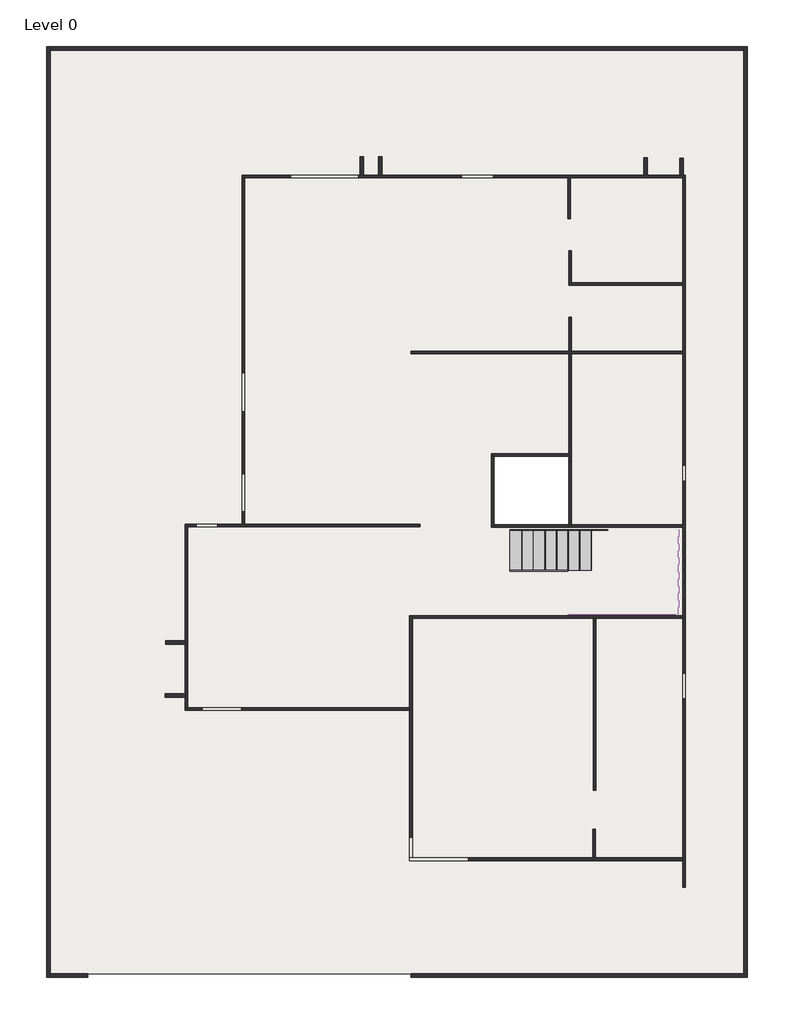
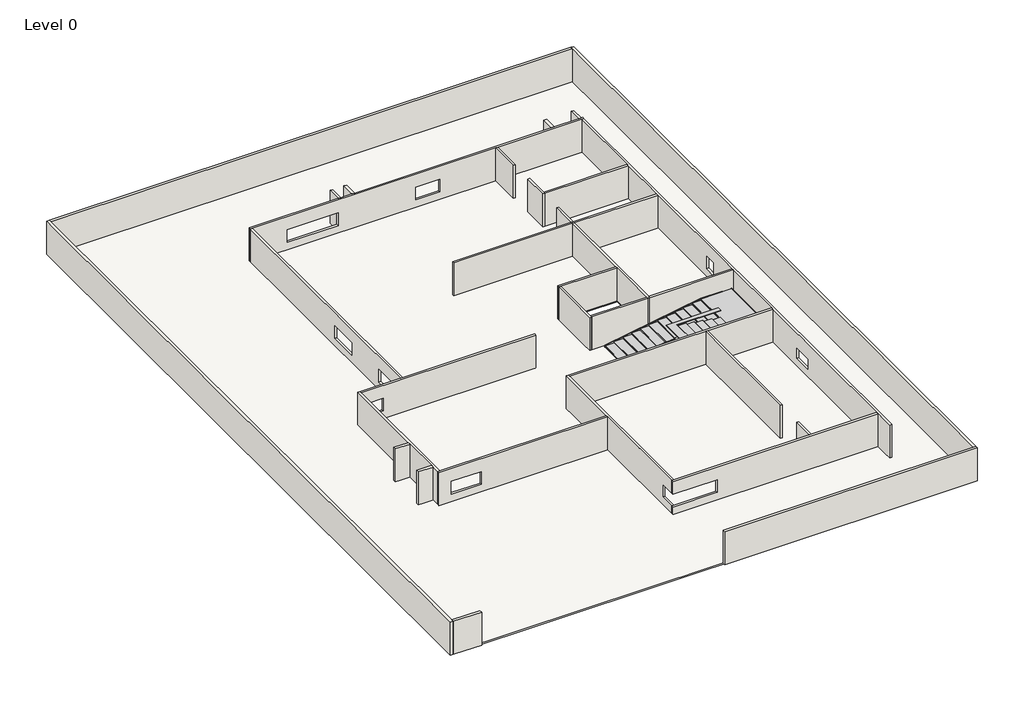
# One storey: 32 walls, 4 members, 1 slab, 1 stair flight.
"""IFC4 building model written with IfcOpenShell, lengths in millimetres."""

from ifc_helpers import new_model, si_unit, frame, origin, origin_with_axes, place, context, project, spatial, polyline, outline, extrude, faceted_brep, transform, mapped, element, save
from components import wood_steps_w_50mm_tread_10mm_nosing_13mm_riser_e98e060e

model = new_model("IFC4")

# Units and contexts
model_context = context("Model", 3, world=origin())
ifc_project = project(units=[si_unit("LENGTHUNIT", "METRE", prefix="MILLI")], contexts=[model_context])

# Site, building, storey
site = spatial("IfcSite", under=ifc_project)
building = spatial("IfcBuilding", under=site)
storey = spatial("IfcBuildingStorey", under=building, Name="Level 0", Elevation=0.0)

# Members
placement = place(None, origin())
element("IfcMember", 1, ObjectType="Stringer-50mm_Width", at=placement, inside=storey, context=model_context, shape_type="SweptSolid", body=[
    extrude(outline(polyline([(193.8557259, -49056.7440401), (0.0, -49056.7440401), (0.0, -47795.0327556), (2042.4365081, -35624.4803934), (2042.4365081, -38041.3469316), (193.8557259, -49056.7440401)])), frame((0.0, 3859.4375818, 0.0), z_axis=(0.0, 1.0, 0.0), x_axis=(0.0, 0.0, 1.0)), (0.0, 0.0, 1.0), 50.0),
])
element("IfcMember", 2, ObjectType="Stringer-50mm_Width", at=placement, inside=storey, context=model_context, shape_type="SweptSolid", body=[
    extrude(outline(polyline([(-34578.7440401, 3909.4375818), (-34528.7440401, 3909.4375818), (-34528.7440401, -3354.1624182), (-34578.7440401, -3354.1624182), (-34578.7440401, 3909.4375818)])), frame((0.0, 0.0, 1642.4365081), z_axis=(0.0, 0.0, 1.0), x_axis=(1.0, 0.0, 0.0)), (0.0, 0.0, 1.0), 400.0),
])
element("IfcMember", 3, ObjectType="Stringer-50mm_Width", at=placement, inside=storey, context=model_context, shape_type="SweptSolid", body=[
    extrude(outline(polyline([(1642.4365081, -34809.0796827), (3197.700045, -44052.9440401), (2792.078062, -44052.9440401), (1642.4365081, -37219.9345007), (1642.4365081, -34809.0796827)])), frame((0.0, -3404.1624182, 0.0), z_axis=(0.0, 1.0, 0.0), x_axis=(0.0, 0.0, 1.0)), (0.0, 0.0, 1.0), 50.0),
])
element("IfcMember", 4, ObjectType="Stringer-50mm_Width", at=placement, inside=storey, context=model_context, shape_type="SweptSolid", body=[
    extrude(outline(polyline([(194.495485, -49056.7440401), (0.0, -49056.7440401), (0.0, -47794.2727754), (625.4624497, -44052.9440401), (1031.0135317, -44052.9440401), (194.495485, -49056.7440401)])), frame((0.0, 362.2005214, 0.0), z_axis=(0.0, 1.0, 0.0), x_axis=(0.0, 0.0, 1.0)), (0.0, 0.0, 1.0), 50.0),
])

# Slab
element("IfcSlab", 5, ObjectType="5\"", at=placement, inside=storey, context=model_context, shape_type="SweptSolid", body=[
    extrude(outline(polyline([(-28918.5480781, 45194.3134919), (-28918.5480781, -34307.6865081), (-88658.4532392, -34307.6865081), (-88658.4532392, 45194.3134919), (-28918.5480781, 45194.3134919)]), holes=[polyline([(-43995.2517152, 10232.8150419), (-50434.1517152, 10232.8150419), (-50434.1517152, 4361.1059175), (-43995.2517152, 4361.1059175), (-43995.2517152, 10232.8150419)])]), frame((0.0, 0.0, -127.0), z_axis=(0.0, 0.0, 1.0), x_axis=(1.0, 0.0, 0.0)), (0.0, 0.0, 1.0), 127.0),
])

# Stair flight
wood_steps_w_50mm_tread_10mm_nosing_13mm_riser_shape = wood_steps_w_50mm_tread_10mm_nosing_13mm_riser_e98e060e(model_context)
element("IfcStairFlight", 6, ObjectType="Wood_Steps_w-50mm_Tread-10mm_Nosing-13mm_Riser", at=placement, inside=storey, context=model_context, shape_type="MappedRepresentation", body=[
    mapped(wood_steps_w_50mm_tread_10mm_nosing_13mm_riser_shape, transform((0.0, 0.0, 0.0), x_axis=(1.0, 0.0, 0.0), y_axis=(0.0, 1.0, 0.0), z_axis=(0.0, 0.0, 1.0))),
])

# Walls
element("IfcWall", 7, ObjectType="12\"", at=placement, inside=storey, context=model_context, shape_type="Brep", body=[
    faceted_brep([(-88963.2532392, 45499.1134919, 0.0), (-88963.2532392, -34612.4865081, 0.0), (-88963.2532392, -34612.4865081, 4000.0), (-88963.2532392, 45499.1134919, 4000.0), (-88658.4532392, 45499.1134919, 0.0), (-88658.4532392, 45499.1134919, 4000.0), (-88658.4532392, 45194.3134919, 4000.0), (-88658.4532392, -34307.6865081, 4000.0), (-88658.4532392, -34612.4865081, 4000.0), (-88658.4532392, -34612.4865081, 0.0), (-88658.4532392, -34307.6865081, 0.0), (-88658.4532392, 45194.3134919, 0.0)], [[[0, 1, 2, 3]], [[4, 5, 6, 7, 8, 9, 10, 11]], [[1, 0, 4, 11, 10, 9]], [[3, 2, 8, 7, 6, 5]], [[0, 3, 5, 4]], [[2, 1, 9, 8]]]),
])
element("IfcWall", 8, ObjectType="12\"", at=placement, inside=storey, context=model_context, shape_type="SweptSolid", body=[
    extrude(outline(polyline([(-85407.2532392, -34612.4865081), (-88658.4532392, -34612.4865081), (-88658.4532392, -34307.6865081), (-85407.2532392, -34307.6865081), (-85407.2532392, -34612.4865081)])), origin_with_axes(), (0.0, 0.0, 1.0), 4000.0),
])
element("IfcWall", 9, ObjectType="12\"", at=placement, inside=storey, context=model_context, shape_type="Brep", body=[
    faceted_brep([(-57569.7480781, -34612.4865081, 0.0), (-28613.7480781, -34612.4865081, 0.0), (-28613.7480781, -34612.4865081, 4000.0), (-57569.7480781, -34612.4865081, 4000.0), (-57569.7480781, -34307.6865081, 0.0), (-57569.7480781, -34307.6865081, 4000.0), (-28918.5480781, -34307.6865081, 4000.0), (-28613.7480781, -34307.6865081, 4000.0), (-28613.7480781, -34307.6865081, 0.0), (-28918.5480781, -34307.6865081, 0.0)], [[[0, 1, 2, 3]], [[4, 5, 6, 7, 8, 9]], [[1, 0, 4, 9, 8]], [[3, 2, 7, 6, 5]], [[0, 3, 5, 4]], [[2, 1, 8, 7]]]),
])
element("IfcWall", 10, ObjectType="12\"", at=placement, inside=storey, context=model_context, shape_type="Brep", body=[
    faceted_brep([(-28613.7480781, -34307.6865081, 0.0), (-28613.7480781, 45499.1134919, 0.0), (-28613.7480781, 45499.1134919, 4000.0), (-28613.7480781, -34307.6865081, 4000.0), (-28918.5480781, -34307.6865081, 0.0), (-28918.5480781, -34307.6865081, 4000.0), (-28918.5480781, 45194.3134919, 4000.0), (-28918.5480781, 45499.1134919, 4000.0), (-28918.5480781, 45499.1134919, 0.0), (-28918.5480781, 45194.3134919, 0.0)], [[[0, 1, 2, 3]], [[4, 5, 6, 7, 8, 9]], [[1, 0, 4, 9, 8]], [[3, 2, 7, 6, 5]], [[2, 1, 8, 7]], [[0, 3, 5, 4]]]),
])
element("IfcWall", 11, ObjectType="12\"", at=placement, inside=storey, context=model_context, shape_type="SweptSolid", body=[
    extrude(outline(polyline([(-88658.4532392, 45499.1134919), (-28918.5480781, 45499.1134919), (-28918.5480781, 45194.3134919), (-88658.4532392, 45194.3134919), (-88658.4532392, 45499.1134919)])), origin_with_axes(), (0.0, 0.0, 1.0), 4000.0),
])
element("IfcWall", 12, ObjectType="12\"", at=placement, inside=storey, context=model_context, shape_type="SweptSolid", body=[
    extrude(outline(polyline([(-61652.3120032, 36022.2059175), (-61652.3120032, 34422.0059175), (-61957.1120032, 34422.0059175), (-61957.1120032, 36022.2059175), (-61652.3120032, 36022.2059175)])), origin_with_axes(), (0.0, 0.0, 1.0), 4000.0),
])
element("IfcWall", 13, ObjectType="12\"", at=placement, inside=storey, context=model_context, shape_type="SweptSolid", body=[
    extrude(outline(polyline([(-60077.5120032, 36022.2059175), (-60077.5120032, 34422.0059175), (-60382.3120032, 34422.0059175), (-60382.3120032, 36022.2059175), (-60077.5120032, 36022.2059175)])), origin_with_axes(), (0.0, 0.0, 1.0), 4000.0),
])
element("IfcWall", 14, ObjectType="12\"", at=placement, inside=storey, context=model_context, shape_type="SweptSolid", body=[
    extrude(outline(polyline([(-37238.8517152, 35920.6059175), (-37238.8517152, 34422.0059175), (-37543.6517152, 34422.0059175), (-37543.6517152, 35920.6059175), (-37238.8517152, 35920.6059175)])), origin_with_axes(), (0.0, 0.0, 1.0), 4000.0),
])
element("IfcWall", 15, ObjectType="12\"", at=placement, inside=storey, context=model_context, shape_type="SweptSolid", body=[
    extrude(outline(polyline([(-34114.6517152, 35895.2059175), (-34114.6517152, 34422.0059175), (-34419.4517152, 34422.0059175), (-34419.4517152, 35895.2059175), (-34114.6517152, 35895.2059175)])), origin_with_axes(), (0.0, 0.0, 1.0), 4000.0),
])
element("IfcWall", 16, ObjectType="12\"", at=placement, inside=storey, context=model_context, shape_type="SweptSolid", body=[
    extrude(outline(polyline([(-78705.700956, -5616.7849581), (-77029.300956, -5616.7849581), (-77029.300956, -5921.5849581), (-78705.700956, -5921.5849581), (-78705.700956, -5616.7849581)])), origin_with_axes(), (0.0, 0.0, 1.0), 4000.0),
])
element("IfcWall", 17, ObjectType="12\"", at=placement, inside=storey, context=model_context, shape_type="SweptSolid", body=[
    extrude(outline(polyline([(-78731.100956, -10188.7849581), (-77029.300956, -10188.7849581), (-77029.300956, -10493.5849581), (-78731.100956, -10493.5849581), (-78731.100956, -10188.7849581)])), origin_with_axes(), (0.0, 0.0, 1.0), 4000.0),
])
element("IfcWall", 18, ObjectType="9\"", at=placement, inside=storey, context=model_context, shape_type="Brep", body=[
    faceted_brep([(-72138.4517152, 34193.4059175, 0.0), (-71909.8517152, 34193.4059175, 0.0), (-44058.7517152, 34193.4059175, 0.0), (-43830.1517152, 34193.4059175, 0.0), (-34190.8517152, 34193.4059175, 0.0), (-33962.2517152, 34193.4059175, 0.0), (-33962.2517152, 34193.4059175, 4000.0), (-34190.8517152, 34193.4059175, 4000.0), (-43830.1517152, 34193.4059175, 4000.0), (-44058.7517152, 34193.4059175, 4000.0), (-71909.8517152, 34193.4059175, 4000.0), (-72138.4517152, 34193.4059175, 4000.0), (-62109.5120032, 34193.4059175, 2438.4), (-62109.5120032, 34193.4059175, 914.4), (-67947.4517152, 34193.4059175, 914.4), (-67947.4517152, 34193.4059175, 2438.4), (-53219.5120032, 34193.4059175, 2438.4), (-50459.5517152, 34193.4059175, 2438.4), (-50459.5517152, 34193.4059175, 914.4), (-53219.5120032, 34193.4059175, 914.4), (-72138.4517152, 34422.0059175, 0.0), (-72138.4517152, 34422.0059175, 4000.0), (-61957.1120032, 34422.0059175, 4000.0), (-61652.3120032, 34422.0059175, 4000.0), (-60382.3120032, 34422.0059175, 4000.0), (-60077.5120032, 34422.0059175, 4000.0), (-37543.6517152, 34422.0059175, 4000.0), (-37238.8517152, 34422.0059175, 4000.0), (-34419.4517152, 34422.0059175, 4000.0), (-34114.6517152, 34422.0059175, 4000.0), (-33962.2517152, 34422.0059175, 4000.0), (-33962.2517152, 34422.0059175, 0.0), (-34114.6517152, 34422.0059175, 0.0), (-34419.4517152, 34422.0059175, 0.0), (-37238.8517152, 34422.0059175, 0.0), (-37543.6517152, 34422.0059175, 0.0), (-60077.5120032, 34422.0059175, 0.0), (-60382.3120032, 34422.0059175, 0.0), (-61652.3120032, 34422.0059175, 0.0), (-61957.1120032, 34422.0059175, 0.0), (-62109.5120032, 34422.0059175, 2438.4), (-67947.4517152, 34422.0059175, 2438.4), (-67947.4517152, 34422.0059175, 914.4), (-62109.5120032, 34422.0059175, 914.4), (-53219.5120032, 34422.0059175, 2438.4), (-53219.5120032, 34422.0059175, 914.4), (-50459.5517152, 34422.0059175, 914.4), (-50459.5517152, 34422.0059175, 2438.4)], [[[0, 1, 2, 3, 4, 5, 6, 7, 8, 9, 10, 11], [12, 13, 14, 15], [16, 17, 18, 19]], [[20, 21, 22, 23, 24, 25, 26, 27, 28, 29, 30, 31, 32, 33, 34, 35, 36, 37, 38, 39], [40, 41, 42, 43], [44, 45, 46, 47]], [[5, 4, 3, 2, 1, 0, 20, 39, 38, 37, 36, 35, 34, 33, 32, 31]], [[11, 10, 9, 8, 7, 6, 30, 29, 28, 27, 26, 25, 24, 23, 22, 21]], [[6, 5, 31, 30]], [[0, 11, 21, 20]], [[13, 12, 40, 43]], [[14, 13, 43, 42]], [[15, 14, 42, 41]], [[12, 15, 41, 40]], [[45, 44, 16, 19]], [[46, 45, 19, 18]], [[47, 46, 18, 17]], [[44, 47, 17, 16]]]),
])
element("IfcWall", 19, ObjectType="9\"", at=placement, inside=storey, context=model_context, shape_type="Brep", body=[
    faceted_brep([(-34190.8517152, 34193.4059175, 0.0), (-34190.8517152, 25176.4059175, 0.0), (-34190.8517152, 24947.8059175, 0.0), (-34190.8517152, 19296.3059175, 0.0), (-34190.8517152, 19067.7059175, 0.0), (-34190.8517152, 4361.1059175, 0.0), (-34190.8517152, 4132.5059175, 0.0), (-34190.8517152, -3474.7940825, 0.0), (-34190.8517152, -3703.3940825, 0.0), (-34190.8517152, -24328.1940825, 0.0), (-34190.8517152, -24556.7940825, 0.0), (-34190.8517152, -26842.7940825, 0.0), (-34190.8517152, -26842.7940825, 4000.0), (-34190.8517152, -24556.7940825, 4000.0), (-34190.8517152, -24328.1940825, 4000.0), (-34190.8517152, -3703.3940825, 4000.0), (-34190.8517152, -3474.7940825, 4000.0), (-34190.8517152, 4132.5059175, 4000.0), (-34190.8517152, 4361.1059175, 4000.0), (-34190.8517152, 19067.7059175, 4000.0), (-34190.8517152, 19296.3059175, 4000.0), (-34190.8517152, 24947.8059175, 4000.0), (-34190.8517152, 25176.4059175, 4000.0), (-34190.8517152, 34193.4059175, 4000.0), (-34190.8517152, 8094.9059175, 2438.4), (-34190.8517152, 8094.9059175, 914.4), (-34190.8517152, 9466.5059175, 914.4), (-34190.8517152, 9466.5059175, 2438.4), (-34190.8517152, -10612.1940825, 2133.6), (-34190.8517152, -10612.1940825, 914.4), (-34190.8517152, -8427.7940825, 914.4), (-34190.8517152, -8427.7940825, 2133.6), (-33962.2517152, 34193.4059175, 0.0), (-33962.2517152, 34193.4059175, 4000.0), (-33962.2517152, -26842.7940825, 4000.0), (-33962.2517152, -26842.7940825, 0.0), (-33962.2517152, 8094.9059175, 2438.4), (-33962.2517152, 9466.5059175, 2438.4), (-33962.2517152, 9466.5059175, 914.4), (-33962.2517152, 8094.9059175, 914.4), (-33962.2517152, -10612.1940825, 2133.6), (-33962.2517152, -8427.7940825, 2133.6), (-33962.2517152, -8427.7940825, 914.4), (-33962.2517152, -10612.1940825, 914.4)], [[[0, 1, 2, 3, 4, 5, 6, 7, 8, 9, 10, 11, 12, 13, 14, 15, 16, 17, 18, 19, 20, 21, 22, 23], [24, 25, 26, 27], [28, 29, 30, 31]], [[32, 33, 34, 35], [36, 37, 38, 39], [40, 41, 42, 43]], [[11, 10, 9, 8, 7, 6, 5, 4, 3, 2, 1, 0, 32, 35]], [[12, 11, 35, 34]], [[23, 22, 21, 20, 19, 18, 17, 16, 15, 14, 13, 12, 34, 33]], [[0, 23, 33, 32]], [[25, 24, 36, 39]], [[26, 25, 39, 38]], [[27, 26, 38, 37]], [[24, 27, 37, 36]], [[29, 28, 40, 43]], [[30, 29, 43, 42]], [[31, 30, 42, 41]], [[28, 31, 41, 40]]]),
])
element("IfcWall", 20, ObjectType="9\"", at=placement, inside=storey, context=model_context, shape_type="Brep", body=[
    faceted_brep([(-34190.8517152, -24328.1940825, 0.0), (-57469.9517152, -24328.1940825, 0.0), (-57698.5517152, -24328.1940825, 0.0), (-57698.5517152, -24328.1940825, 914.4), (-57469.9517152, -24328.1940825, 914.4), (-52631.2517152, -24328.1940825, 914.4), (-52631.2517152, -24328.1940825, 2438.4), (-57469.9517152, -24328.1940825, 2438.4), (-57698.5517152, -24328.1940825, 2438.4), (-57698.5517152, -24328.1940825, 4000.0), (-57469.9517152, -24328.1940825, 4000.0), (-34190.8517152, -24328.1940825, 4000.0), (-57698.5517152, -24556.7940825, 0.0), (-34190.8517152, -24556.7940825, 0.0), (-34190.8517152, -24556.7940825, 4000.0), (-57698.5517152, -24556.7940825, 4000.0), (-57698.5517152, -24556.7940825, 2438.4), (-52631.2517152, -24556.7940825, 2438.4), (-52631.2517152, -24556.7940825, 914.4), (-57698.5517152, -24556.7940825, 914.4)], [[[0, 1, 2, 3, 4, 5, 6, 7, 8, 9, 10, 11]], [[12, 13, 14, 15, 16, 17, 18, 19]], [[2, 1, 0, 13, 12]], [[11, 10, 9, 15, 14]], [[0, 11, 14, 13]], [[2, 12, 19, 3]], [[15, 9, 8, 16]], [[3, 19, 18, 5, 4]], [[6, 17, 16, 8, 7]], [[17, 6, 5, 18]]]),
])
element("IfcWall", 21, ObjectType="9\"", at=placement, inside=storey, context=model_context, shape_type="Brep", body=[
    faceted_brep([(-57469.9517152, -24328.1940825, 0.0), (-57469.9517152, -3703.3940825, 0.0), (-57469.9517152, -3474.7940825, 0.0), (-57469.9517152, -3474.7940825, 4000.0), (-57469.9517152, -3703.3940825, 4000.0), (-57469.9517152, -24328.1940825, 4000.0), (-57469.9517152, -24328.1940825, 2438.4), (-57469.9517152, -22550.1940825, 2438.4), (-57469.9517152, -22550.1940825, 914.4), (-57469.9517152, -24328.1940825, 914.4), (-57698.5517152, -3474.7940825, 0.0), (-57698.5517152, -11407.9849581, 0.0), (-57698.5517152, -11636.5849581, 0.0), (-57698.5517152, -24328.1940825, 0.0), (-57698.5517152, -24328.1940825, 914.4), (-57698.5517152, -22550.1940825, 914.4), (-57698.5517152, -22550.1940825, 2438.4), (-57698.5517152, -24328.1940825, 2438.4), (-57698.5517152, -24328.1940825, 4000.0), (-57698.5517152, -11636.5849581, 4000.0), (-57698.5517152, -11407.9849581, 4000.0), (-57698.5517152, -3474.7940825, 4000.0)], [[[0, 1, 2, 3, 4, 5, 6, 7, 8, 9]], [[10, 11, 12, 13, 14, 15, 16, 17, 18, 19, 20, 21]], [[2, 1, 0, 13, 12, 11, 10]], [[5, 4, 3, 21, 20, 19, 18]], [[5, 18, 17, 6]], [[13, 0, 9, 14]], [[3, 2, 10, 21]], [[8, 15, 14, 9]], [[15, 8, 7, 16]], [[16, 7, 6, 17]]]),
])
element("IfcWall", 22, ObjectType="9\"", at=placement, inside=storey, context=model_context, shape_type="SweptSolid", body=[
    extrude(outline(polyline([(-34190.8517152, -3703.3940825), (-57469.9517152, -3703.3940825), (-57469.9517152, -3474.7940825), (-34190.8517152, -3474.7940825), (-34190.8517152, -3703.3940825)])), origin_with_axes(), (0.0, 0.0, 1.0), 4000.0),
])
element("IfcWall", 23, ObjectType="9\"", at=placement, inside=storey, context=model_context, shape_type="SweptSolid", body=[
    extrude(outline(polyline([(-41877.4094181, -18486.1940825), (-41877.4094181, -3703.3940825), (-41648.8094181, -3703.3940825), (-41648.8094181, -18486.1940825), (-41877.4094181, -18486.1940825)])), origin_with_axes(), (0.0, 0.0, 1.0), 4000.0),
])
element("IfcWall", 24, ObjectType="9\"", at=placement, inside=storey, context=model_context, shape_type="SweptSolid", body=[
    extrude(outline(polyline([(-41911.3593333, -24328.1940825), (-41911.3593333, -21852.3403847), (-41682.7593333, -21852.3403847), (-41682.7593333, -24328.1940825), (-41911.3593333, -24328.1940825)])), origin_with_axes(), (0.0, 0.0, 1.0), 4000.0),
])
element("IfcWall", 25, ObjectType="9\"", at=placement, inside=storey, context=model_context, shape_type="SweptSolid", body=[
    extrude(outline(polyline([(34193.4059175, 0.0), (4403.5150419, 0.0), (4403.5150419, 4000.0), (34193.4059175, 4000.0), (34193.4059175, 0.0)]), holes=[polyline([(5470.3150419, 2438.4), (5470.3150419, 914.4), (8742.6059175, 914.4), (8742.6059175, 2438.4), (5470.3150419, 2438.4)]), polyline([(17429.4059175, 2438.4), (14076.6059175, 2438.4), (14076.6059175, 914.4), (17429.4059175, 914.4), (17429.4059175, 2438.4)])]), frame((-72138.4517152, 0.0, 0.0), z_axis=(1.0, 0.0, 0.0), x_axis=(0.0, 1.0, 0.0)), (0.0, 0.0, 1.0), 228.6),
])
element("IfcWall", 26, ObjectType="9\"", at=placement, inside=storey, context=model_context, shape_type="SweptSolid", body=[
    extrude(outline(polyline([(0.0, -76800.700956), (0.0, -56798.200956), (4000.0, -56798.200956), (4000.0, -76800.700956), (0.0, -76800.700956)]), holes=[polyline([(2438.4, -74248.000956), (914.4, -74248.000956), (914.4, -76089.500956), (2438.4, -76089.500956), (2438.4, -74248.000956)])]), frame((0.0, 4174.9150419, 0.0), z_axis=(0.0, 1.0, 0.0), x_axis=(0.0, 0.0, 1.0)), (0.0, 0.0, 1.0), 228.6),
])
element("IfcWall", 27, ObjectType="9\"", at=placement, inside=storey, context=model_context, shape_type="Brep", body=[
    faceted_brep([(-77029.300956, 4403.5150419, 0.0), (-77029.300956, -5616.7849581, 0.0), (-77029.300956, -5921.5849581, 0.0), (-77029.300956, -10188.7849581, 0.0), (-77029.300956, -10493.5849581, 0.0), (-77029.300956, -11407.9849581, 0.0), (-77029.300956, -11407.9849581, 4000.0), (-77029.300956, -10493.5849581, 4000.0), (-77029.300956, -10188.7849581, 4000.0), (-77029.300956, -5921.5849581, 4000.0), (-77029.300956, -5616.7849581, 4000.0), (-77029.300956, 4403.5150419, 4000.0), (-76800.700956, 4403.5150419, 0.0), (-76800.700956, 4403.5150419, 4000.0), (-76800.700956, 4174.9150419, 4000.0), (-76800.700956, -11407.9849581, 4000.0), (-76800.700956, -11407.9849581, 0.0), (-76800.700956, 4174.9150419, 0.0)], [[[0, 1, 2, 3, 4, 5, 6, 7, 8, 9, 10, 11]], [[12, 13, 14, 15, 16, 17]], [[5, 4, 3, 2, 1, 0, 12, 17, 16]], [[11, 10, 9, 8, 7, 6, 15, 14, 13]], [[6, 5, 16, 15]], [[0, 11, 13, 12]]]),
])
element("IfcWall", 28, ObjectType="9\"", at=placement, inside=storey, context=model_context, shape_type="Brep", body=[
    faceted_brep([(-77029.300956, -11636.5849581, 0.0), (-57698.5517152, -11636.5849581, 0.0), (-57698.5517152, -11636.5849581, 4000.0), (-77029.300956, -11636.5849581, 4000.0), (-75581.500956, -11636.5849581, 2438.4), (-72176.5517152, -11636.5849581, 2438.4), (-72176.5517152, -11636.5849581, 914.4), (-75581.500956, -11636.5849581, 914.4), (-77029.300956, -11407.9849581, 0.0), (-77029.300956, -11407.9849581, 4000.0), (-76800.700956, -11407.9849581, 4000.0), (-57698.5517152, -11407.9849581, 4000.0), (-57698.5517152, -11407.9849581, 0.0), (-76800.700956, -11407.9849581, 0.0), (-75581.500956, -11407.9849581, 2438.4), (-75581.500956, -11407.9849581, 914.4), (-72176.5517152, -11407.9849581, 914.4), (-72176.5517152, -11407.9849581, 2438.4)], [[[0, 1, 2, 3], [4, 5, 6, 7]], [[8, 9, 10, 11, 12, 13], [14, 15, 16, 17]], [[1, 0, 8, 13, 12]], [[3, 2, 11, 10, 9]], [[2, 1, 12, 11]], [[0, 3, 9, 8]], [[15, 14, 4, 7]], [[16, 15, 7, 6]], [[17, 16, 6, 5]], [[14, 17, 5, 4]]]),
])
element("IfcWall", 29, ObjectType="9\"", at=placement, inside=storey, context=model_context, shape_type="Brep", body=[
    faceted_brep([(-34190.8517152, 19296.3059175, 0.0), (-43766.6517152, 19296.3059175, 0.0), (-43995.2517152, 19296.3059175, 0.0), (-57596.9517152, 19296.3059175, 0.0), (-57596.9517152, 19296.3059175, 4000.0), (-43995.2517152, 19296.3059175, 4000.0), (-43766.6517152, 19296.3059175, 4000.0), (-34190.8517152, 19296.3059175, 4000.0), (-34190.8517152, 19067.7059175, 0.0), (-34190.8517152, 19067.7059175, 4000.0), (-43766.6517152, 19067.7059175, 4000.0), (-43995.2517152, 19067.7059175, 4000.0), (-57596.9517152, 19067.7059175, 4000.0), (-57596.9517152, 19067.7059175, 0.0), (-43995.2517152, 19067.7059175, 0.0), (-43766.6517152, 19067.7059175, 0.0)], [[[0, 1, 2, 3, 4, 5, 6, 7]], [[8, 9, 10, 11, 12, 13, 14, 15]], [[3, 2, 1, 0, 8, 15, 14, 13]], [[4, 3, 13, 12]], [[7, 6, 5, 4, 12, 11, 10, 9]], [[0, 7, 9, 8]]]),
])
element("IfcWall", 30, ObjectType="9\"", at=placement, inside=storey, context=model_context, shape_type="SweptSolid", body=[
    extrude(outline(polyline([(-43766.6517152, 22191.9059175), (-43766.6517152, 19296.3059175), (-43995.2517152, 19296.3059175), (-43995.2517152, 22191.9059175), (-43766.6517152, 22191.9059175)])), origin_with_axes(), (0.0, 0.0, 1.0), 4000.0),
])
element("IfcWall", 31, ObjectType="9\"", at=placement, inside=storey, context=model_context, shape_type="Brep", body=[
    faceted_brep([(-43995.2517152, 19067.7059175, 0.0), (-43995.2517152, 10461.4150419, 0.0), (-43995.2517152, 10232.8150419, 0.0), (-43995.2517152, 4361.1059175, 0.0), (-43995.2517152, 4132.5059175, 0.0), (-43995.2517152, 4132.5059175, 4000.0), (-43995.2517152, 4361.1059175, 4000.0), (-43995.2517152, 10232.8150419, 4000.0), (-43995.2517152, 10461.4150419, 4000.0), (-43995.2517152, 19067.7059175, 4000.0), (-43766.6517152, 19067.7059175, 0.0), (-43766.6517152, 19067.7059175, 4000.0), (-43766.6517152, 4361.1059175, 4000.0), (-43766.6517152, 4132.5059175, 4000.0), (-43766.6517152, 4132.5059175, 0.0), (-43766.6517152, 4361.1059175, 0.0)], [[[0, 1, 2, 3, 4, 5, 6, 7, 8, 9]], [[10, 11, 12, 13, 14, 15]], [[4, 3, 2, 1, 0, 10, 15, 14]], [[9, 8, 7, 6, 5, 13, 12, 11]], [[0, 9, 11, 10]], [[5, 4, 14, 13]]]),
])
element("IfcWall", 32, ObjectType="9\"", at=placement, inside=storey, context=model_context, shape_type="SweptSolid", body=[
    extrude(outline(polyline([(-34190.8517152, 4132.5059175), (-43766.6517152, 4132.5059175), (-43766.6517152, 4361.1059175), (-34190.8517152, 4361.1059175), (-34190.8517152, 4132.5059175)])), origin_with_axes(), (0.0, 0.0, 1.0), 4000.0),
])
element("IfcWall", 33, ObjectType="9\"", at=placement, inside=storey, context=model_context, shape_type="Brep", body=[
    faceted_brep([(-43995.2517152, 10461.4150419, 0.0), (-50662.7517152, 10461.4150419, 0.0), (-50662.7517152, 10461.4150419, 4000.0), (-43995.2517152, 10461.4150419, 4000.0), (-43995.2517152, 10232.8150419, 0.0), (-43995.2517152, 10232.8150419, 4000.0), (-50434.1517152, 10232.8150419, 4000.0), (-50662.7517152, 10232.8150419, 4000.0), (-50662.7517152, 10232.8150419, 0.0), (-50434.1517152, 10232.8150419, 0.0)], [[[0, 1, 2, 3]], [[4, 5, 6, 7, 8, 9]], [[1, 0, 4, 9, 8]], [[3, 2, 7, 6, 5]], [[0, 3, 5, 4]], [[2, 1, 8, 7]]]),
])
element("IfcWall", 34, ObjectType="9\"", at=placement, inside=storey, context=model_context, shape_type="Brep", body=[
    faceted_brep([(-50662.7517152, 10232.8150419, 0.0), (-50662.7517152, 4132.5059175, 0.0), (-50662.7517152, 4132.5059175, 4000.0), (-50662.7517152, 10232.8150419, 4000.0), (-50434.1517152, 10232.8150419, 0.0), (-50434.1517152, 10232.8150419, 4000.0), (-50434.1517152, 4361.1059175, 4000.0), (-50434.1517152, 4132.5059175, 4000.0), (-50434.1517152, 4132.5059175, 0.0), (-50434.1517152, 4361.1059175, 0.0)], [[[0, 1, 2, 3]], [[4, 5, 6, 7, 8, 9]], [[1, 0, 4, 9, 8]], [[3, 2, 7, 6, 5]], [[0, 3, 5, 4]], [[2, 1, 8, 7]]]),
])
element("IfcWall", 35, ObjectType="9\"", at=placement, inside=storey, context=model_context, shape_type="SweptSolid", body=[
    extrude(outline(polyline([(-43995.2517152, 4132.5059175), (-50434.1517152, 4132.5059175), (-50434.1517152, 4361.1059175), (-43995.2517152, 4361.1059175), (-43995.2517152, 4132.5059175)])), origin_with_axes(), (0.0, 0.0, 1.0), 4000.0),
])
element("IfcWall", 36, ObjectType="9\"", at=placement, inside=storey, context=model_context, shape_type="SweptSolid", body=[
    extrude(outline(polyline([(-44058.7517152, 30675.5059175), (-44058.7517152, 34193.4059175), (-43830.1517152, 34193.4059175), (-43830.1517152, 30675.5059175), (-44058.7517152, 30675.5059175)])), origin_with_axes(), (0.0, 0.0, 1.0), 4000.0),
])
element("IfcWall", 37, ObjectType="9\"", at=placement, inside=storey, context=model_context, shape_type="Brep", body=[
    faceted_brep([(-43995.2517152, 27932.3059175, 0.0), (-43995.2517152, 24947.8059175, 0.0), (-43995.2517152, 24947.8059175, 4000.0), (-43995.2517152, 27932.3059175, 4000.0), (-43766.6517152, 27932.3059175, 0.0), (-43766.6517152, 27932.3059175, 4000.0), (-43766.6517152, 25176.4059175, 4000.0), (-43766.6517152, 24947.8059175, 4000.0), (-43766.6517152, 24947.8059175, 0.0), (-43766.6517152, 25176.4059175, 0.0)], [[[0, 1, 2, 3]], [[4, 5, 6, 7, 8, 9]], [[1, 0, 4, 9, 8]], [[3, 2, 7, 6, 5]], [[0, 3, 5, 4]], [[2, 1, 8, 7]]]),
])
element("IfcWall", 38, ObjectType="9\"", at=placement, inside=storey, context=model_context, shape_type="SweptSolid", body=[
    extrude(outline(polyline([(-34190.8517152, 24947.8059175), (-43766.6517152, 24947.8059175), (-43766.6517152, 25176.4059175), (-34190.8517152, 25176.4059175), (-34190.8517152, 24947.8059175)])), origin_with_axes(), (0.0, 0.0, 1.0), 4000.0),
])

save(model, "model.ifc")

# Revit data of these elements
# Type "5\""
#   Keynote = "E60/130"
#   Function = 0
#   Layers, outside or top first: 0' - 5" "Concrete, Precast" (function 1)
# Type "12\""
#   Layers, outside or top first: 1' - 0" "Concrete Masonry Units" (function 1)
# Type "9\""
#   Layers, outside or top first: 0' - 9" "Concrete Masonry Units" (function 1)
# Elements 1, 2, 3, 4 (IfcMember, "Stringer-50mm_Width")
#   Phase Created = New Construction
# Element 5 (IfcSlab, "5\"")
#   Height Offset From Level = 0' - 0"
#   Phase Created = New Construction
#   Materials on its faces: "Concrete, Precast"
# Element 6 (IfcStairFlight, "Wood_Steps_w-50mm_Tread-10mm_Nosing-13mm_Riser")
#   Phase Created = New Construction
#   Materials on its faces: "Oak Flooring"
# Elements 7, 8, 9, 10, 11, 12, 13, 14, 15, 16, 17 (IfcWall, "12\"")
#   Top Offset = 0' - 0"
#   Base Offset = 0' - 0"
#   wall height = 13' - 1.48031"
#   Phase Created = New Construction
#   Base Constraint = Level 0
#   Top Constraint = Level 1
#   Materials on its faces: "Concrete Masonry Units"
# Elements 18, 19, 20, 21, 22, 23, 24, 25, 26, 27, 28, 29, 30, 31, 32, 33, 34, 35, 36, 37, 38 (IfcWall, "9\"")
#   Top Offset = 0' - 0"
#   Base Offset = 0' - 0"
#   wall height = 13' - 1.48031"
#   Phase Created = New Construction
#   Base Constraint = Level 0
#   Top Constraint = Level 1
#   Materials on its faces: "Concrete Masonry Units"
# Materials
#   "Concrete, Precast": class "Concrete", colour RGB 192 192 192, transparency 0, Description = "Precast concrete", Cost = 0
#   "Concrete Masonry Units": class "Masonry", colour RGB 181 181 181, transparency 0, Description = "Concrete masonry units", Cost = 0
#   "Oak Flooring": class "Wood", colour RGB 212 179 113, transparency 0, Description = "Quercus Rubra", Cost = 0
